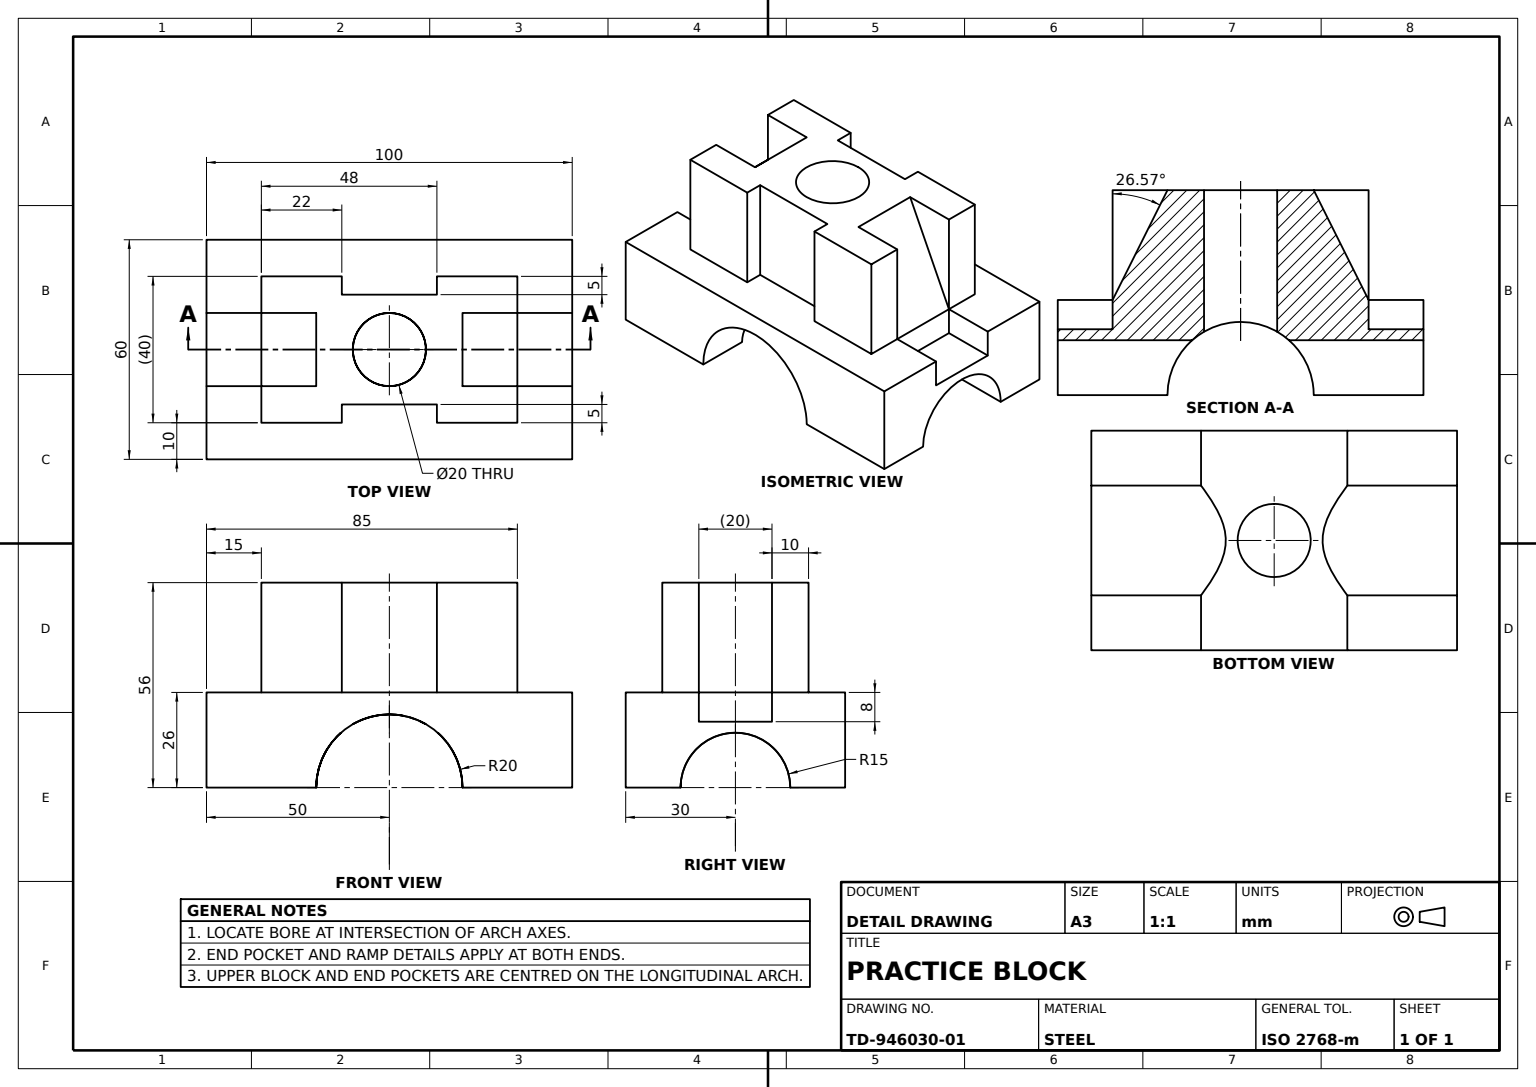
SolidWorks part; units mm, degrees
material "Plain Carbon Steel"
ref_plane "Front Plane" through (0, 0, 0) normal (0, 0, 1) x (1, 0, 0)
ref_plane "Top Plane" through (0, 0, 0) normal (0, 1, 0) x (1, 0, 0)
ref_plane "Right Plane" through (0, 0, 0) normal (1, 0, 0) x (0, 0, -1)
sketch "Base Profile Sketch" plane through (0, 0, 0) normal (0, 1, 0) x (1, 0, 0)
  line L1 (50, 0) -> (50, 30)
  line L2 (50, 30) -> (-50, 30)
  line L3 (-50, 30) -> (-50, -30)
  line L4 (-50, -30) -> (50, -30)
  line L5 (50, -30) -> (50, 0)
  dimension "D1" = 100
  dimension "D2" = 60
  dimension "D3" = 30
  dimension "D4" = 50
extrude "Base Block" add sketch "Base Profile Sketch" along normal blind 26
sketch "Upper Block Sketch" plane through (0, 26, 0) normal (0, 1, 0) x (1, 0, 0)
  line L0 (50, -30) -> (50, 30) construction
  line L1 (35, 0) -> (35, 20)
  line L2 (35, 20) -> (-35, 20)
  line L3 (-35, 20) -> (-35, -20)
  line L4 (-35, -20) -> (35, -20)
  line L5 (35, -20) -> (35, 0)
  line L6 (50, 30) -> (-50, 30) construction
  dimension "D1" = 15
  dimension "D2" = 85
  dimension "D3" = 10
  dimension "D4" = 30
extrude "Upper Guide Block" add sketch "Upper Block Sketch" along normal blind 30
sketch "Guide Slots Sketch" plane through (0, 56, 0) normal (0, 1, 0) x (1, 0, 0)
  line L0 (35, 0) -> (35, 10)
  line L1 (35, -20) -> (35, 20) construction
  line L2 (35, 10) -> (20, 10)
  line L3 (20, 10) -> (20, -10)
  line L4 (20, -10) -> (35, -10)
  line L5 (35, -20) -> (35, 20) construction
  line L8 (-35, -20) -> (35, -20) construction
  line L9 (13, -20) -> (13, -15)
  line L10 (13, -15) -> (-13, -15)
  line L11 (-13, -15) -> (-13, -20)
  line L12 (-35, -20) -> (35, -20) construction
  line L15 (-35, 20) -> (-35, -20) construction
  line L16 (-35, -10) -> (-20, -10)
  line L17 (-20, -10) -> (-20, 10)
  line L18 (-20, 10) -> (-35, 10)
  line L21 (35, 20) -> (-35, 20) construction
  line L22 (-13, 20) -> (-13, 15)
  line L23 (-13, 15) -> (13, 15)
  line L24 (13, 15) -> (13, 20)
  line L27 (-13, 20) -> (13, 20)
  line L28 (35, 0) -> (35, -10)
  line L29 (-13, -20) -> (13, -20)
  line L30 (-35, 10) -> (-35, -10)
  line L31 (35, 20) -> (-35, 20) construction
  dimension "D1" = 15
  dimension "D2" = 22
  dimension "D3" = 48
  dimension "D4" = 5
  dimension "D5" = 10
extrude "Guide Slots Cut" cut sketch "Guide Slots Sketch" against normal blind 30
ref_plane "Boss Offset Plane" through (0, 0, 10) normal (0, 0, 1) x (1, 0, 0)
sketch "Offset Boss Sketch" plane through (0, 0, 10) normal (0, 0, 1) x (1, 0, 0)
  line L1 (-35, 56) -> (-13, 56) construction
  line L2 (-20, 56) -> (-35, 26)
  line L3 (-35, 26) -> (-20, 26)
  line L4 (-50, 26) -> (50, 26) construction
  line L5 (-20, 26) -> (-20, 56)
  line L7 (13, 56) -> (35, 56) construction
  line L8 (20, 56) -> (35, 26)
  line L9 (35, 26) -> (20, 26)
  line L10 (20, 26) -> (20, 56)
  dimension "D1" = 40
extrude "Offset Boss" add sketch "Offset Boss Sketch" against normal blind 20
sketch "Top Bore Sketch" plane through (0, 56, 0) normal (0, 1, 0) x (1, 0, 0)
  circle A0 centre (0, 0) radius 10
  dimension "D1" = 20
extrude "Top Bore" cut sketch "Top Bore Sketch" against normal blind 83
sketch "Pocket Sketch" plane through (0, 26, 0) normal (0, 1, 0) x (1, 0, 0)
  line L0 (35, 10) -> (50, 10)
  line L1 (50, -30) -> (50, 30) construction
  line L2 (50, 10) -> (50, -10)
  line L3 (50, -10) -> (35, -10)
  line L4 (35, -10) -> (35, 10)
  line L5 (-35, 10) -> (-50, 10)
  line L6 (-50, 30) -> (-50, -30) construction
  line L7 (-50, 10) -> (-50, -10)
  line L8 (-50, -10) -> (-35, -10)
  line L9 (-35, -10) -> (-35, 10)
extrude "Pocket 8mm Deep" cut sketch "Pocket Sketch" against normal blind 8
sketch "Side Arch Sketch" plane through (-50, 0, 0) normal (-1, 0, 0) x (0, 0, 1)
  line L0 (-30, 0) -> (30, 0) construction
  line L1 (-15, 0) -> (15, 0)
  arc A0 (15, 0) -> (-15, 0) centre (0, 0) ccw
  dimension "D1" = 15
extrude "Side Arch Cut" cut sketch "Side Arch Sketch" against normal blind 121
sketch "Bearing Arch Sketch" plane through (0, 0, -30) normal (0, 0, -1) x (-1, 0, 0)
  circle A0 centre (0, 0) radius 20
  dimension "D1" = 40
extrude "Bearing Arch Cut" cut sketch "Bearing Arch Sketch" against normal blind 121
